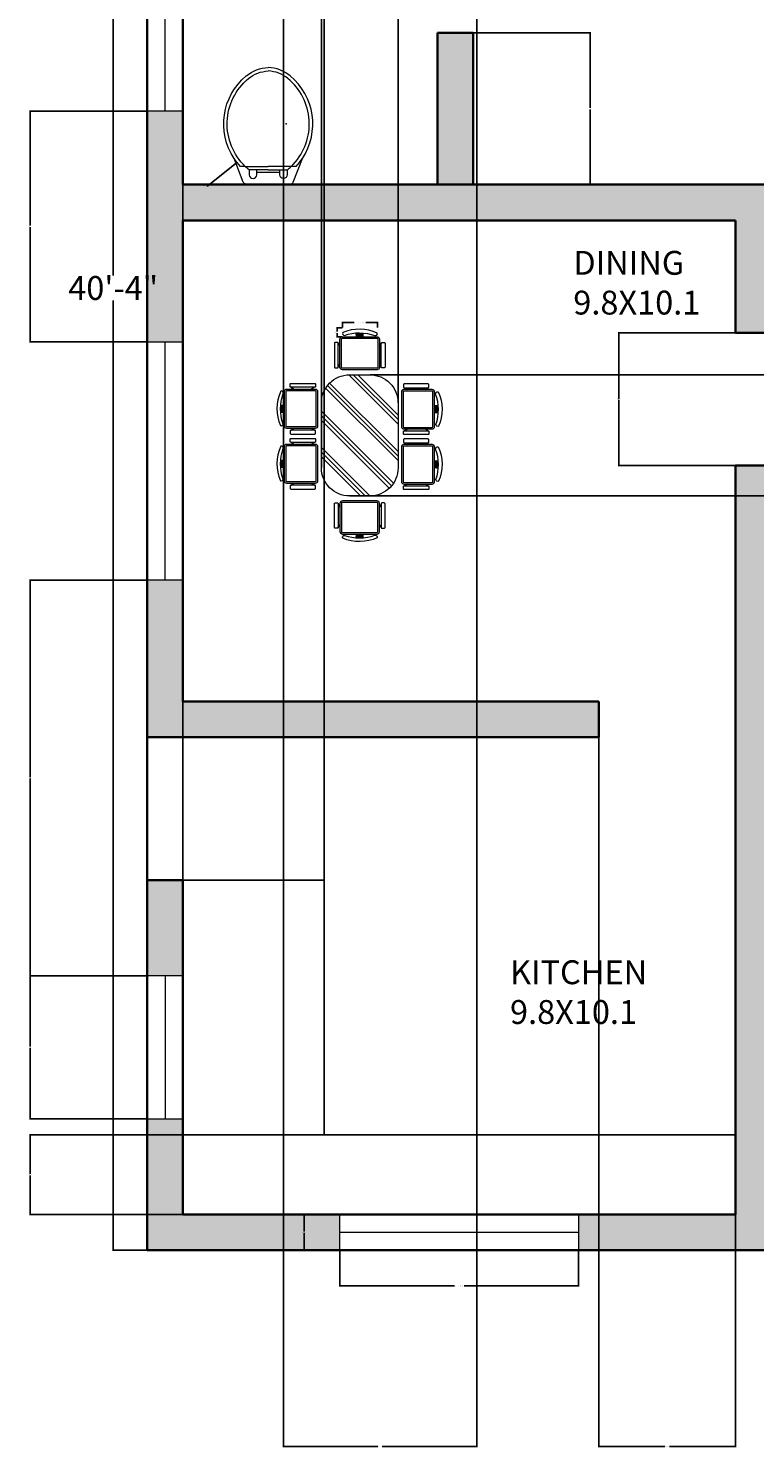
# Model space of a CAD drawing. Units: inches. Extents: x 0 to 423, y -517 to 94.
# Tile 1 of 8: x 0 to 182, y -517 to -160. Entities that reach past the tile are written whole.
import ezdxf

# ---------------------------------------------------------------- set-up
doc = ezdxf.new("R2010")
doc.units = ezdxf.units.IN
doc.header["$MEASUREMENT"] = 0
for name, color, linetype, lineweight in [('A-ANNO-DIMS', 2, 'Continuous', 18), ('A-AREA-IDEN', 7, 'Continuous', 18), ('A-FLOR-CASE', 8, 'Continuous', 25), ('A-FURN', 8, 'Continuous', 13), ('A-FURN-PATT', 8, 'Continuous', 13), ('A-GLAZ', 4, 'Continuous', 18), ('A-WALL', 7, 'Continuous', 35), ('WC-Detail_dwgmodels.com', 251, 'Continuous', 13), ('WC-Outline_dwgmodels.com', 250, 'Continuous', 18)]:
    doc.layers.add(name, color=color, linetype=linetype, lineweight=lineweight)
doc.layers.add('A-WALL-PATT', color=30, linetype='Continuous', lineweight=13, true_color=0xf26722)
doc.styles.get("Standard").update_dxf_attribs({"font": 'arial.ttf'})
doc.dimstyles.get("Standard").update_dxf_attribs({"dimtxt": 0.18, "dimasz": 0.18, "dimexe": 0.18, "dimexo": 0.0625, "dimgap": 0.09, "dimtad": 0, "dimtih": 1, "dimtoh": 1, "dimdec": 0, "dimzin": 0, "dimdsep": 46, "dimlunit": 3, "dimtxsty": 'Standard', "dimcen": 0.09, "dimadec": 0, "dimazin": 0, "dimtfac": 1, "dimtdec": 0, "dimtofl": 0, "dimtmove": 0, "dimatfit": 3, "dimfxl": 1, "dimtolj": 1, "dimtzin": 0, "dimarcsym": 0})

# ---------------------------------------------------------------- blocks, each defined once
blk = doc.blocks.new('*D2')
at = {"layer": 'A-ANNO-DIMS', "color": 0, "lineweight": -2, "transparency": 16777216}
for p, q in [((29.66, 16.23), (21, 16.23)), ((21.18, 16.05), (21.18, -222.61)), ((21.18, -467.59), (21.18, -228.92)), ((29.66, -467.77), (21, -467.77))]:
    blk.add_line(p, q, dxfattribs=at)
at = {"layer": 'A-ANNO-DIMS', "color": 0, "transparency": 16777216}
for points in [[(21.15, 16.05), (21.21, 16.05), (21.18, 16.23)], [(21.15, -467.59), (21.21, -467.59), (21.18, -467.77)]]:
    blk.add_solid(points, dxfattribs=at)
at = {"layer": 'Defpoints', "color": 0, "transparency": 16777216}
for p in [(29.72, 16.23), (21.18, -467.77), (29.72, -467.77)]:
    blk.add_point(p, dxfattribs=at)
at = {"layer": 'A-ANNO-DIMS', "color": 0, "transparency": 16777216, "insert": (21.18, -225.77), "char_height": 6, "attachment_point": 5}
blk.add_mtext('\\A1;40\'-4"', dxfattribs=at)
blk = doc.blocks.new('WIN-GLAZ-60IN')
for p, q in [((0, 60), (0, 0)), ((4.5, 60), (4.5, 0)), ((9, 0), (9, 60))]:
    blk.add_line(p, q)
blk = doc.blocks.new('WIN-GLAZ-24IN')
for p, q in [((0, 0), (0, 24)), ((4.5, 0), (4.5, 24)), ((9, 24), (9, 0))]:
    blk.add_line(p, q)
blk = doc.blocks.new('DINING-CHAIR-BACKREST')
for p, q in [((3.29, 0.7), (5.3, 0.7)), ((3.31, 0.47), (5.3, 0.47)), ((3.31, 0.2), (5.3, 0.2))]:
    blk.add_line(p, q)
blk.add_lwpolyline([(0.05, 1.03, 0.552014), (0.46, 0.34, -0.175809), (8.12, 0.28, 0.578392), (8.7, 0.92, 0.214524)], format="xyb", close=True)
blk.add_lwpolyline([(4.3, 0), (4.3, 0.93)])
blk = doc.blocks.new('*D12')
at = {"layer": 'A-ANNO-DIMS', "color": 0, "lineweight": -2, "transparency": 16777216}
for p, q in [((78.22, -467.83), (78.22, -476.95)), ((138.22, -467.83), (138.22, -476.95)), ((78.4, -476.77), (106.99, -476.77)), ((138.04, -476.77), (109.45, -476.77))]:
    blk.add_line(p, q, dxfattribs=at)
at = {"layer": 'A-ANNO-DIMS', "color": 0, "transparency": 16777216}
for points in [[(78.4, -476.74), (78.4, -476.8), (78.22, -476.77)], [(138.04, -476.74), (138.04, -476.8), (138.22, -476.77)]]:
    blk.add_solid(points, dxfattribs=at)
at = {"layer": 'Defpoints', "color": 0, "transparency": 16777216}
for p in [(78.22, -467.77), (138.22, -467.77), (78.22, -476.77)]:
    blk.add_point(p, dxfattribs=at)
at = {"layer": 'A-ANNO-DIMS', "color": 0, "transparency": 16777216, "insert": (108.22, -476.77), "char_height": 0.18, "attachment_point": 5}
blk.add_mtext('\\A1;WINDOW 5\'-0" TYP.', dxfattribs=at)
blk = doc.blocks.new('*D13')
at = {"layer": 'A-ANNO-DIMS', "color": 0, "lineweight": -2, "transparency": 16777216}
for p, q in [((78.16, -458.77), (69.04, -458.77)), ((69.22, -458.95), (69.22, -463.08)), ((69.22, -467.59), (69.22, -463.45)), ((78.16, -467.77), (69.04, -467.77))]:
    blk.add_line(p, q, dxfattribs=at)
at = {"layer": 'A-ANNO-DIMS', "color": 0, "transparency": 16777216}
for points in [[(69.19, -458.95), (69.25, -458.95), (69.22, -458.77)], [(69.19, -467.59), (69.25, -467.59), (69.22, -467.77)]]:
    blk.add_solid(points, dxfattribs=at)
at = {"layer": 'Defpoints', "color": 0, "transparency": 16777216}
for p in [(69.22, -458.77), (78.22, -458.77), (78.22, -467.77)]:
    blk.add_point(p, dxfattribs=at)
at = {"layer": 'A-ANNO-DIMS', "color": 0, "transparency": 16777216, "insert": (69.22, -463.27), "char_height": 0.18, "attachment_point": 5}
blk.add_mtext('\\A1;0\'-9" TYP.', dxfattribs=at)
blk = doc.blocks.new('*D16')
at = {"layer": 'A-ANNO-DIMS', "color": 0, "lineweight": -2, "transparency": 16777216}
for p, q in [((78.85, -235.73), (78.85, -234.3)), ((79.03, -234.48), (81.8, -234.48)), ((87.45, -234.48), (84.68, -234.48)), ((87.63, -235.73), (87.63, -234.3))]:
    blk.add_line(p, q, dxfattribs=at)
at = {"layer": 'A-ANNO-DIMS', "color": 0, "transparency": 16777216}
for points in [[(79.03, -234.45), (79.03, -234.51), (78.85, -234.48)], [(87.45, -234.45), (87.45, -234.51), (87.63, -234.48)]]:
    blk.add_solid(points, dxfattribs=at)
at = {"layer": 'Defpoints', "color": 0, "transparency": 16777216}
for p in [(87.63, -234.48), (78.85, -235.8), (87.63, -235.8)]:
    blk.add_point(p, dxfattribs=at)
at = {"layer": 'A-ANNO-DIMS', "color": 0, "transparency": 16777216, "insert": (83.24, -234.48), "char_height": 0.18, "attachment_point": 5}
blk.add_mtext('\\A1;CHAIR BACK 0\'-9" TYP.', dxfattribs=at)
blk = doc.blocks.new('*D17')
at = {"layer": 'A-ANNO-DIMS', "color": 0, "lineweight": -2, "transparency": 16777216}
for p, q in [((78.79, -235.8), (77.36, -235.8)), ((78.79, -238.03), (77.36, -238.03)), ((77.54, -235.98), (77.54, -236.73)), ((77.54, -237.85), (77.54, -237.09))]:
    blk.add_line(p, q, dxfattribs=at)
at = {"layer": 'A-ANNO-DIMS', "color": 0, "transparency": 16777216}
for points in [[(77.51, -235.98), (77.57, -235.98), (77.54, -235.8)], [(77.51, -237.85), (77.57, -237.85), (77.54, -238.03)]]:
    blk.add_solid(points, dxfattribs=at)
at = {"layer": 'Defpoints', "color": 0, "transparency": 16777216}
for p in [(77.54, -235.8), (78.85, -235.8), (78.85, -238.03)]:
    blk.add_point(p, dxfattribs=at)
at = {"layer": 'A-ANNO-DIMS', "color": 0, "transparency": 16777216, "insert": (77.54, -236.91), "char_height": 0.18, "attachment_point": 5}
blk.add_mtext('\\A1;0\'-2" TYP.', dxfattribs=at)
blk = doc.blocks.new('*D33')
at = {"layer": 'A-ANNO-DIMS', "color": 0, "lineweight": -2, "transparency": 16777216}
for p, q in [((38.72, -374.65), (38.72, 45.81)), ((38.9, 45.63), (55.89, 45.63)), ((74.1, 45.63), (57.11, 45.63)), ((74.28, -374.65), (74.28, 45.81))]:
    blk.add_line(p, q, dxfattribs=at)
at = {"layer": 'A-ANNO-DIMS', "color": 0, "transparency": 16777216}
for points in [[(38.9, 45.66), (38.9, 45.6), (38.72, 45.63)], [(74.1, 45.66), (74.1, 45.6), (74.28, 45.63)]]:
    blk.add_solid(points, dxfattribs=at)
at = {"layer": 'Defpoints', "color": 0, "transparency": 16777216}
for p in [(74.28, 45.63), (38.72, -374.71), (74.28, -374.71)]:
    blk.add_point(p, dxfattribs=at)
at = {"layer": 'A-ANNO-DIMS', "color": 0, "transparency": 16777216, "insert": (56.5, 45.63), "char_height": 0.18, "attachment_point": 5}
blk.add_mtext('\\A1;2\'-11 1/2"', dxfattribs=at)
blk = doc.blocks.new('*D34')
at = {"layer": 'A-ANNO-DIMS', "color": 0, "lineweight": -2, "transparency": 16777216}
for p, q in [((74.21, -438.77), (0.14, -438.77)), ((0.32, -438.95), (0.32, -448.59)), ((0.32, -458.59), (0.32, -448.95)), ((38.66, -458.77), (0.14, -458.77))]:
    blk.add_line(p, q, dxfattribs=at)
at = {"layer": 'A-ANNO-DIMS', "color": 0, "transparency": 16777216}
for points in [[(0.29, -438.95), (0.35, -438.95), (0.32, -438.77)], [(0.29, -458.59), (0.35, -458.59), (0.32, -458.77)]]:
    blk.add_solid(points, dxfattribs=at)
at = {"layer": 'Defpoints', "color": 0, "transparency": 16777216}
for p in [(0.32, -438.77), (74.28, -438.77), (38.72, -458.77)]:
    blk.add_point(p, dxfattribs=at)
at = {"layer": 'A-ANNO-DIMS', "color": 0, "transparency": 16777216, "insert": (0.32, -448.77), "char_height": 0.18, "attachment_point": 5}
blk.add_mtext('\\A1;1\'-8"', dxfattribs=at)
blk = doc.blocks.new('*D46')
at = {"layer": 'A-ANNO-DIMS', "color": 0, "lineweight": -2, "transparency": 16777216}
for p, q in [((29.66, -181.27), (0.14, -181.27)), ((0.32, -181.45), (0.32, -210.08)), ((0.32, -239.09), (0.32, -210.45)), ((29.66, -239.27), (0.14, -239.27))]:
    blk.add_line(p, q, dxfattribs=at)
at = {"layer": 'A-ANNO-DIMS', "color": 0, "transparency": 16777216}
for points in [[(0.29, -181.45), (0.35, -181.45), (0.32, -181.27)], [(0.29, -239.09), (0.35, -239.09), (0.32, -239.27)]]:
    blk.add_solid(points, dxfattribs=at)
at = {"layer": 'Defpoints', "color": 0, "transparency": 16777216}
for p in [(0.32, -181.27), (29.72, -181.27), (29.72, -239.27)]:
    blk.add_point(p, dxfattribs=at)
at = {"layer": 'A-ANNO-DIMS', "color": 0, "transparency": 16777216, "insert": (0.32, -210.27), "char_height": 0.18, "attachment_point": 5}
blk.add_mtext('\\A1;4\'-10"', dxfattribs=at)
blk = doc.blocks.new('*D47')
at = {"layer": 'A-ANNO-DIMS', "color": 0, "lineweight": -2, "transparency": 16777216}
for p, q in [((29.66, -299.27), (0.14, -299.27)), ((0.32, -299.45), (0.32, -348.82)), ((0.32, -398.56), (0.32, -349.18)), ((29.66, -398.74), (0.14, -398.74))]:
    blk.add_line(p, q, dxfattribs=at)
at = {"layer": 'A-ANNO-DIMS', "color": 0, "transparency": 16777216}
for points in [[(0.29, -299.45), (0.35, -299.45), (0.32, -299.27)], [(0.29, -398.56), (0.35, -398.56), (0.32, -398.74)]]:
    blk.add_solid(points, dxfattribs=at)
at = {"layer": 'Defpoints', "color": 0, "transparency": 16777216}
for p in [(0.32, -299.27), (29.72, -299.27), (29.72, -398.74)]:
    blk.add_point(p, dxfattribs=at)
at = {"layer": 'A-ANNO-DIMS', "color": 0, "transparency": 16777216, "insert": (0.32, -349), "char_height": 0.18, "attachment_point": 5}
blk.add_mtext('\\A1;8\'-3 1/2"', dxfattribs=at)
blk = doc.blocks.new('*D48')
at = {"layer": 'A-ANNO-DIMS', "color": 0, "lineweight": -2, "transparency": 16777216}
for p, q in [((29.66, -398.74), (0.14, -398.74)), ((0.32, -398.92), (0.32, -416.55)), ((0.32, -434.56), (0.32, -416.92)), ((29.66, -434.74), (0.14, -434.74))]:
    blk.add_line(p, q, dxfattribs=at)
at = {"layer": 'A-ANNO-DIMS', "color": 0, "transparency": 16777216}
for points in [[(0.29, -398.92), (0.35, -398.92), (0.32, -398.74)], [(0.29, -434.56), (0.35, -434.56), (0.32, -434.74)]]:
    blk.add_solid(points, dxfattribs=at)
at = {"layer": 'Defpoints', "color": 0, "transparency": 16777216}
for p in [(0.32, -398.74), (29.72, -398.74), (29.72, -434.74)]:
    blk.add_point(p, dxfattribs=at)
at = {"layer": 'A-ANNO-DIMS', "color": 0, "transparency": 16777216, "insert": (0.32, -416.74), "char_height": 0.18, "attachment_point": 5}
blk.add_mtext('\\A1;3\'-0"', dxfattribs=at)
blk = doc.blocks.new('*D49')
at = {"layer": 'A-ANNO-DIMS', "color": 0, "lineweight": -2, "transparency": 16777216}
for p, q in [((63.98, -61.2), (63.98, -517.35)), ((112.6, -61.2), (112.6, -517.35)), ((64.16, -517.17), (87.75, -517.17)), ((112.42, -517.17), (88.83, -517.17))]:
    blk.add_line(p, q, dxfattribs=at)
at = {"layer": 'A-ANNO-DIMS', "color": 0, "transparency": 16777216}
for points in [[(64.16, -517.14), (64.16, -517.2), (63.98, -517.17)], [(112.42, -517.14), (112.42, -517.2), (112.6, -517.17)]]:
    blk.add_solid(points, dxfattribs=at)
at = {"layer": 'Defpoints', "color": 0, "transparency": 16777216}
for p in [(63.98, -61.14), (112.6, -61.14), (112.6, -517.17)]:
    blk.add_point(p, dxfattribs=at)
at = {"layer": 'A-ANNO-DIMS', "color": 0, "transparency": 16777216, "insert": (88.29, -517.17), "char_height": 0.18, "attachment_point": 5}
blk.add_mtext('\\A1;4\'-0 1/2"', dxfattribs=at)
blk = doc.blocks.new('*D52')
at = {"layer": 'A-ANNO-DIMS', "color": 0, "lineweight": -2, "transparency": 16777216}
for p, q in [((73.55, -270.94), (73.55, 45.81)), ((73.73, 45.63), (82.66, 45.63)), ((92.66, 45.63), (83.72, 45.63)), ((92.84, -254.62), (92.84, 45.81))]:
    blk.add_line(p, q, dxfattribs=at)
at = {"layer": 'A-ANNO-DIMS', "color": 0, "transparency": 16777216}
for points in [[(73.73, 45.66), (73.73, 45.6), (73.55, 45.63)], [(92.66, 45.66), (92.66, 45.6), (92.84, 45.63)]]:
    blk.add_solid(points, dxfattribs=at)
at = {"layer": 'Defpoints', "color": 0, "transparency": 16777216}
for p in [(92.84, 45.63), (92.84, -254.68), (73.55, -271)]:
    blk.add_point(p, dxfattribs=at)
at = {"layer": 'A-ANNO-DIMS', "color": 0, "transparency": 16777216, "insert": (83.19, 45.63), "char_height": 0.18, "attachment_point": 5}
blk.add_mtext('\\A1;1\'-7 1/2"', dxfattribs=at)
blk = doc.blocks.new('*D53')
at = {"layer": 'A-ANNO-DIMS', "color": 0, "lineweight": -2, "transparency": 16777216}
for p, q in [((85.83, -247.61), (422.3, -247.61)), ((422.12, -247.79), (422.12, -262.66)), ((422.12, -277.89), (422.12, -263.02)), ((80.68, -278.07), (422.3, -278.07))]:
    blk.add_line(p, q, dxfattribs=at)
at = {"layer": 'A-ANNO-DIMS', "color": 0, "transparency": 16777216}
for points in [[(422.09, -247.79), (422.15, -247.79), (422.12, -247.61)], [(422.09, -277.89), (422.15, -277.89), (422.12, -278.07)]]:
    blk.add_solid(points, dxfattribs=at)
at = {"layer": 'Defpoints', "color": 0, "transparency": 16777216}
for p in [(85.77, -247.61), (80.61, -278.07), (422.12, -278.07)]:
    blk.add_point(p, dxfattribs=at)
at = {"layer": 'A-ANNO-DIMS', "color": 0, "transparency": 16777216, "insert": (422.12, -262.84), "char_height": 0.18, "attachment_point": 5}
blk.add_mtext('\\A1;2\'-6 1/2"', dxfattribs=at)
blk = doc.blocks.new('*D54')
at = {"layer": 'A-ANNO-DIMS', "color": 0, "lineweight": -2, "transparency": 16777216}
for p, q in [((177.72, -270.44), (177.72, -517.35)), ((143.29, -338.83), (143.29, -517.35)), ((143.47, -517.17), (159.9, -517.17)), ((177.54, -517.17), (161.12, -517.17))]:
    blk.add_line(p, q, dxfattribs=at)
at = {"layer": 'A-ANNO-DIMS', "color": 0, "transparency": 16777216}
for points in [[(143.47, -517.14), (143.47, -517.2), (143.29, -517.17)], [(177.54, -517.14), (177.54, -517.2), (177.72, -517.17)]]:
    blk.add_solid(points, dxfattribs=at)
at = {"layer": 'Defpoints', "color": 0, "transparency": 16777216}
for p in [(177.72, -270.38), (143.29, -338.77), (177.72, -517.17)]:
    blk.add_point(p, dxfattribs=at)
at = {"layer": 'A-ANNO-DIMS', "color": 0, "transparency": 16777216, "insert": (160.51, -517.17), "char_height": 0.18, "attachment_point": 5}
blk.add_mtext('\\A1;2\'-10 1/2"', dxfattribs=at)
blk = doc.blocks.new('*D56')
at = {"layer": 'A-ANNO-DIMS', "color": 0, "lineweight": -2, "transparency": 16777216}
for p, q in [((177.66, -237.07), (148.14, -237.07)), ((148.32, -237.25), (148.32, -253.54)), ((148.32, -270.2), (148.32, -253.91)), ((177.66, -270.38), (148.14, -270.38))]:
    blk.add_line(p, q, dxfattribs=at)
at = {"layer": 'A-ANNO-DIMS', "color": 0, "transparency": 16777216}
for points in [[(148.29, -237.25), (148.35, -237.25), (148.32, -237.07)], [(148.29, -270.2), (148.35, -270.2), (148.32, -270.38)]]:
    blk.add_solid(points, dxfattribs=at)
at = {"layer": 'Defpoints', "color": 0, "transparency": 16777216}
for p in [(148.32, -237.07), (177.72, -237.07), (177.72, -270.38)]:
    blk.add_point(p, dxfattribs=at)
at = {"layer": 'A-ANNO-DIMS', "color": 0, "transparency": 16777216, "insert": (148.32, -253.72), "char_height": 0.18, "attachment_point": 5}
blk.add_mtext('\\A1;2\'-9 1/2"', dxfattribs=at)
blk = doc.blocks.new('*D57')
at = {"layer": 'A-ANNO-DIMS', "color": 0, "lineweight": -2, "transparency": 16777216}
for p, q in [((111.79, -161.55), (141.3, -161.55)), ((141.12, -161.73), (141.12, -180.47)), ((141.12, -199.59), (141.12, -180.84)), ((111.79, -199.77), (141.3, -199.77))]:
    blk.add_line(p, q, dxfattribs=at)
at = {"layer": 'A-ANNO-DIMS', "color": 0, "transparency": 16777216}
for points in [[(141.09, -161.73), (141.15, -161.73), (141.12, -161.55)], [(141.09, -199.59), (141.15, -199.59), (141.12, -199.77)]]:
    blk.add_solid(points, dxfattribs=at)
at = {"layer": 'Defpoints', "color": 0, "transparency": 16777216}
for p in [(111.72, -161.55), (111.72, -199.77), (141.12, -199.77)]:
    blk.add_point(p, dxfattribs=at)
at = {"layer": 'A-ANNO-DIMS', "color": 0, "transparency": 16777216, "insert": (141.12, -180.66), "char_height": 0.18, "attachment_point": 5}
blk.add_mtext('\\A1;3\'-2"', dxfattribs=at)
blk = doc.blocks.new('*D67')
at = {"layer": 'A-ANNO-DIMS', "color": 0, "lineweight": -2, "transparency": 16777216}
for p, q in [((64.56, -184.51), (64.74, -184.51)), ((64.65, -184.6), (64.65, -184.42)), ((44.95, -200.04), (52.2, -194.33)), ((44.77, -200.04), (44.95, -200.04))]:
    blk.add_line(p, q, dxfattribs=at)
at = {"layer": 'A-ANNO-DIMS', "color": 0, "transparency": 16777216}
blk.add_solid([(52.18, -194.31), (52.22, -194.35), (52.34, -194.22)], dxfattribs=at)
at = {"layer": 'Defpoints', "color": 0, "transparency": 16777216}
for p in [(64.65, -184.51), (52.34, -194.22)]:
    blk.add_point(p, dxfattribs=at)
at = {"layer": 'A-ANNO-DIMS', "color": 0, "transparency": 16777216, "insert": (44.15, -200.04), "char_height": 0.18, "attachment_point": 5}
blk.add_mtext('\\A1;R1\'-3 1/2"', dxfattribs=at)

msp = doc.modelspace()

# ---------------------------------------------------------------- hatches: boundary and pattern name
at = {"layer": 'A-FURN-PATT'}
h = msp.add_hatch(dxfattribs=at)
h.set_pattern_fill('PLAST', color=256, scale=25.912, angle=135, style=0)
h.paths.add_polyline_path([(85.77, -278.07), (80.61, -278.07), (80.25, -278.06), (79.89, -278.03), (79.54, -277.98), (79.19, -277.92), (78.85, -277.84), (78.51, -277.75), (78.18, -277.64), (77.86, -277.51), (77.55, -277.37), (77.25, -277.21), (76.95, -277.04), (76.66, -276.86), (76.39, -276.66), (76.12, -276.45), (75.86, -276.23), (75.62, -276), (75.38, -275.75), (75.16, -275.49), (74.95, -275.23), (74.75, -274.95), (74.57, -274.66), (74.4, -274.37), (74.24, -274.06), (74.1, -273.75), (73.98, -273.43), (73.87, -273.1), (73.77, -272.77), (73.69, -272.42), (73.63, -272.08), (73.58, -271.72), (73.56, -271.36), (73.55, -271), (73.55, -254.68), (73.56, -254.32), (73.58, -253.96), (73.63, -253.6), (73.69, -253.25), (73.77, -252.91), (73.87, -252.58), (73.98, -252.25), (74.1, -251.93), (74.24, -251.61), (74.4, -251.31), (74.57, -251.01), (74.75, -250.73), (74.95, -250.45), (75.16, -250.18), (75.38, -249.93), (75.62, -249.68), (75.86, -249.45), (76.12, -249.23), (76.39, -249.02), (76.66, -248.82), (76.95, -248.63), (77.25, -248.46), (77.55, -248.31), (77.86, -248.17), (78.18, -248.04), (78.51, -247.93), (78.85, -247.83), (79.19, -247.76), (79.54, -247.69), (79.89, -247.65), (80.25, -247.62), (80.61, -247.61), (85.77, -247.61), (86.13, -247.62), (86.49, -247.65), (86.85, -247.69), (87.2, -247.76), (87.54, -247.83), (87.87, -247.93), (88.2, -248.04), (88.52, -248.17), (88.83, -248.31), (89.14, -248.46), (89.44, -248.63), (89.72, -248.82), (90, -249.02), (90.27, -249.23), (90.52, -249.45), (90.77, -249.68), (91, -249.93), (91.22, -250.18), (91.43, -250.45), (91.63, -250.73), (91.81, -251.01), (91.99, -251.31), (92.14, -251.61), (92.28, -251.93), (92.41, -252.25), (92.52, -252.58), (92.62, -252.91), (92.69, -253.25), (92.76, -253.6), (92.8, -253.96), (92.83, -254.32), (92.84, -254.68), (92.84, -271), (92.83, -271.35), (92.8, -271.7), (92.76, -272.04), (92.7, -272.38), (92.62, -272.72), (92.53, -273.05), (92.42, -273.38), (92.3, -273.7), (92.16, -274.02), (92.01, -274.33), (91.84, -274.63), (91.65, -274.92), (91.45, -275.2), (91.24, -275.48), (91.01, -275.74), (90.77, -276), (90.51, -276.24), (90.25, -276.47), (89.98, -276.68), (89.69, -276.88), (89.4, -277.06), (89.1, -277.23), (88.79, -277.39), (88.48, -277.53), (88.15, -277.65), (87.83, -277.76), (87.49, -277.85), (87.16, -277.93), (86.81, -277.99), (86.47, -278.03), (86.12, -278.06)])
at = {"layer": 'A-WALL-PATT'}
h = msp.add_hatch(color=256, dxfattribs=at)
h.dxf.hatch_style = 1
h.paths.add_polyline_path([(201.52, 16.23), (138.22, 16.23), (138.22, 7.23), (177.72, 7.23), (177.72, -138.77), (186.72, -138.77), (186.72, -92.77), (251.72, -92.77), (251.72, -22.53), (242.72, -22.53), (242.72, -83.77), (186.72, -83.77), (186.72, 7.23), (201.52, 7.23)])
h.paths.add_polyline_path([(78.22, 16.23), (29.72, 16.23), (29.72, -31.27), (38.72, -31.27), (38.72, 7.23), (78.22, 7.23)])
h.paths.add_polyline_path([(275.31, 16.23), (225.52, 16.23), (225.52, 7.23), (275.31, 7.23)])
h.paths.add_polyline_path([(392.72, 16.23), (335.31, 16.23), (335.31, 7.23), (383.72, 7.23), (383.72, -31.27), (392.72, -31.27)])
h.paths.add_polyline_path([(143.33, -129.77), (38.72, -129.77), (38.72, -91.27), (29.72, -91.27), (29.72, -157.27), (38.72, -157.27), (38.72, -138.77), (143.33, -138.77)])
h.paths.add_polyline_path([(186.72, -199.77), (38.72, -199.77), (38.72, -181.27), (29.72, -181.27), (29.72, -239.27), (38.72, -239.27), (38.72, -208.77), (177.72, -208.77), (177.72, -237.07), (186.72, -237.07)])
h.paths.add_polyline_path([(111.72, -161.55), (102.72, -161.55), (102.72, -199.77), (111.72, -199.77)])
h.paths.add_polyline_path([(392.72, -91.27), (383.72, -91.27), (383.72, -129.77), (242.72, -129.77), (242.72, -138.77), (383.72, -138.77), (383.72, -169.77), (392.72, -169.77)])
h.paths.add_polyline_path([(392.72, -229.77), (383.72, -229.77), (383.72, -262.77), (251.72, -262.77), (251.72, -177.14), (242.72, -177.14), (242.72, -271.77), (383.72, -271.77), (383.72, -300.77), (392.72, -300.77)])
h.paths.add_polyline_path([(392.72, -360.77), (383.72, -360.77), (383.72, -389.77), (378.42, -389.77), (378.42, -398.77), (383.72, -398.77), (383.72, -458.77), (382.72, -458.77), (382.72, -467.77), (392.72, -467.77)])
h.paths.add_polyline_path([(364.92, -389.77), (348.72, -389.77), (348.72, -467.77), (358.72, -467.77), (358.72, -458.77), (357.72, -458.77), (357.72, -398.77), (364.92, -398.77)])
h.paths.add_polyline_path([(320.72, -389.77), (283.72, -389.77), (283.72, -398.77), (320.72, -398.77)])
h.paths.add_polyline_path([(223.72, -389.77), (186.72, -389.77), (186.72, -270.38), (177.72, -270.38), (177.72, -458.77), (138.22, -458.77), (138.22, -467.77), (186.72, -467.77), (186.72, -398.77), (223.72, -398.77)])
h.paths.add_polyline_path([(143.29, -329.77), (38.72, -329.77), (38.72, -299.27), (29.72, -299.27), (29.72, -338.77), (143.29, -338.77)])
h.paths.add_polyline_path([(38.72, -374.71), (29.72, -374.71), (29.72, -398.74), (38.72, -398.74)])
h.paths.add_polyline_path([(78.22, -458.77), (38.72, -458.77), (38.72, -434.74), (29.72, -434.74), (29.72, -467.77), (78.22, -467.77)])
h.paths.add_polyline_path([(279.99, -158.17), (326.6, -158.17), (326.6, -135.78), (279.99, -135.78)], flags=25)
h.paths.add_polyline_path([(355.56, -439.13), (387, -439.13), (387, -416.66), (355.56, -416.66)], flags=9)

# ---------------------------------------------------------------- linework, layer by layer
at = {"layer": 'A-FLOR-CASE'}
for p, q in [((38.72, -374.71), (74.28, -374.71)), ((74.28, -374.71), (74.28, -438.77)), ((74.28, -438.77), (177.72, -438.77))]:
    msp.add_line(p, q, dxfattribs=at)
at = {"layer": 'A-FURN'}
for p, q in [((77.79, -239.74), (78.21, -240.26)), ((88.57, -239.74), (88.14, -240.26)), ((77.79, -245.58), (78.21, -244.88)), ((88.57, -245.58), (88.14, -244.88)), ((65.96, -250.74), (66.48, -251.17)), ((71.8, -250.74), (71.1, -251.17)), ((94.45, -250.88), (95.15, -251.31)), ((100.29, -250.88), (99.76, -251.31)), ((65.96, -261.53), (66.48, -261.1)), ((71.8, -261.53), (71.1, -261.1)), ((94.45, -261.66), (95.15, -261.24)), ((100.29, -261.66), (99.76, -261.24)), ((65.96, -264.58), (66.48, -265.01)), ((71.8, -264.58), (71.1, -265.01)), ((94.45, -264.72), (95.15, -265.15)), ((100.29, -264.72), (99.76, -265.15)), ((65.96, -275.37), (66.48, -274.94)), ((71.8, -275.37), (71.1, -274.94)), ((94.45, -275.5), (95.15, -275.08)), ((100.29, -275.5), (99.76, -275.08)), ((77.79, -280.1), (78.21, -280.8)), ((88.57, -280.1), (88.14, -280.8)), ((77.79, -285.94), (78.21, -285.42)), ((88.57, -285.94), (88.14, -285.42))]:
    msp.add_line(p, q, dxfattribs=at)
for points in [[(88.13, -238.62), (88.13, -245.76, -0.414214), (87.54, -246.35), (78.82, -246.35, -0.414214), (78.22, -245.76), (78.22, -238.62, -0.414214), (78.82, -238.03)], [(78.82, -238.03), (87.54, -238.03, -0.414214), (88.13, -238.62)], [(89.35, -239.49, -0.414214), (89.55, -239.69), (89.55, -245.64, -0.414214), (89.35, -245.83), (88.76, -245.83, -0.414214), (88.56, -245.64), (88.56, -239.69, -0.414214)], [(88.56, -239.69, -0.414214), (88.76, -239.49), (89.35, -239.49, -0.414214)], [(65.71, -249.96, -0.414214), (65.91, -249.76), (71.86, -249.76, -0.414214), (72.06, -249.96), (72.06, -250.55, -0.414214), (71.86, -250.75), (65.91, -250.75, -0.414214)], [(64.84, -251.18), (71.98, -251.18, -0.414214), (72.58, -251.77), (72.58, -260.5, -0.414214), (71.98, -261.09), (64.84, -261.09, -0.414214), (64.25, -260.5)], [(64.25, -260.5), (64.25, -251.77, -0.414214), (64.84, -251.18)], [(65.91, -250.75, -0.414214), (65.71, -250.55), (65.71, -249.96, -0.414214)], [(102, -251.91, 0.414214), (101.4, -251.32), (94.27, -251.32, 0.414214), (93.67, -251.91), (93.67, -260.63, 0.414214), (94.27, -261.23), (101.4, -261.23, 0.414214), (102, -260.63)], [(100.54, -250.1, 0.414214), (100.34, -249.9), (94.39, -249.9, 0.414214), (94.19, -250.1), (94.19, -250.69, 0.414214), (94.39, -250.89), (100.34, -250.89, 0.414214)], [(100.34, -250.89, 0.414214), (100.54, -250.69), (100.54, -250.1, 0.414214)], [(102, -260.63), (102, -251.91, 0.414214)], [(65.71, -263.8, -0.414214), (65.91, -263.6), (71.86, -263.6, -0.414214), (72.06, -263.8), (72.06, -264.39, -0.414214), (71.86, -264.59), (65.91, -264.59, -0.414214)], [(65.91, -264.59, -0.414214), (65.71, -264.39), (65.71, -263.8, -0.414214)], [(100.54, -263.94, 0.414214), (100.34, -263.74), (94.39, -263.74, 0.414214), (94.19, -263.94), (94.19, -264.53, 0.414214), (94.39, -264.73), (100.34, -264.73, 0.414214)], [(100.34, -264.73, 0.414214), (100.54, -264.53), (100.54, -263.94, 0.414214)], [(64.84, -265.02), (71.98, -265.02, -0.414214), (72.58, -265.61), (72.58, -274.34, -0.414214), (71.98, -274.93), (64.84, -274.93, -0.414214), (64.25, -274.34)], [(64.25, -274.34), (64.25, -265.61, -0.414214), (64.84, -265.02)], [(102, -265.75, 0.414214), (101.4, -265.16), (94.27, -265.16, 0.414214), (93.67, -265.75), (93.67, -274.47, 0.414214), (94.27, -275.07), (101.4, -275.07, 0.414214), (102, -274.47)], [(102, -274.47), (102, -265.75, 0.414214)], [(87.54, -287.65, 0.414214), (88.13, -287.06), (88.13, -279.92, 0.414214), (87.54, -279.32), (78.82, -279.32, 0.414214), (78.22, -279.92), (78.22, -287.06, 0.414214), (78.82, -287.65)], [(89.35, -286.19, 0.414214), (89.55, -285.99), (89.55, -280.04, 0.414214), (89.35, -279.84), (88.76, -279.84, 0.414214), (88.56, -280.04), (88.56, -285.99, 0.414214)], [(78.82, -287.65), (87.54, -287.65, 0.414214)], [(88.56, -285.99, 0.414214), (88.76, -286.19), (89.35, -286.19, 0.414214)]]:
    msp.add_lwpolyline(points, format="xyb", dxfattribs=at)
for points in [[(78.82, -238.42), (87.54, -238.42, -0.414214), (87.74, -238.62), (87.74, -245.76, -0.414214), (87.54, -245.96), (78.82, -245.96, -0.414214), (78.62, -245.76), (78.62, -238.62, -0.414214)], [(77.6, -239.49), (77, -239.49, 0.414214), (76.8, -239.69), (76.8, -245.64, 0.414214), (77, -245.83), (77.6, -245.83, 0.414214), (77.79, -245.64), (77.79, -239.69, 0.414214)], [(85.77, -278.07), (80.61, -278.07, -0.414214), (73.55, -271), (73.55, -254.68, -0.414214), (80.61, -247.61), (85.77, -247.61, -0.414214), (92.84, -254.68), (92.84, -271, -0.414214)], [(64.65, -260.5), (64.65, -251.77, -0.414214), (64.84, -251.58), (71.98, -251.58, -0.414214), (72.18, -251.77), (72.18, -260.5, -0.414214), (71.98, -260.7), (64.84, -260.7, -0.414214)], [(101.6, -260.63), (101.6, -251.91, 0.414214), (101.4, -251.71), (94.27, -251.71, 0.414214), (94.07, -251.91), (94.07, -260.63, 0.414214), (94.27, -260.83), (101.4, -260.83, 0.414214)], [(65.71, -261.72), (65.71, -262.31, 0.414214), (65.91, -262.51), (71.86, -262.51, 0.414214), (72.06, -262.31), (72.06, -261.72, 0.414214), (71.86, -261.52), (65.91, -261.52, 0.414214)], [(100.54, -261.85), (100.54, -262.45, -0.414214), (100.34, -262.65), (94.39, -262.65, -0.414214), (94.19, -262.45), (94.19, -261.85, -0.414214), (94.39, -261.66), (100.34, -261.66, -0.414214)], [(64.65, -274.34), (64.65, -265.61, -0.414214), (64.84, -265.42), (71.98, -265.42, -0.414214), (72.18, -265.61), (72.18, -274.34, -0.414214), (71.98, -274.53), (64.84, -274.53, -0.414214)], [(101.6, -274.47), (101.6, -265.75, 0.414214), (101.4, -265.55), (94.27, -265.55, 0.414214), (94.07, -265.75), (94.07, -274.47, 0.414214), (94.27, -274.67), (101.4, -274.67, 0.414214)], [(65.71, -275.56), (65.71, -276.15, 0.414214), (65.91, -276.35), (71.86, -276.35, 0.414214), (72.06, -276.15), (72.06, -275.56, 0.414214), (71.86, -275.36), (65.91, -275.36, 0.414214)], [(100.54, -275.69), (100.54, -276.29, -0.414214), (100.34, -276.49), (94.39, -276.49, -0.414214), (94.19, -276.29), (94.19, -275.69, -0.414214), (94.39, -275.5), (100.34, -275.5, -0.414214)], [(77.6, -286.19), (77, -286.19, -0.414214), (76.8, -285.99), (76.8, -280.04, -0.414214), (77, -279.84), (77.6, -279.84, -0.414214), (77.79, -280.04), (77.79, -285.99, -0.414214)], [(78.82, -287.25), (87.54, -287.25, 0.414214), (87.74, -287.06), (87.74, -279.92, 0.414214), (87.54, -279.72), (78.82, -279.72, 0.414214), (78.62, -279.92), (78.62, -287.06, 0.414214)]]:
    msp.add_lwpolyline(points, format="xyb", close=True, dxfattribs=at)
for points in [[(77.59, -239.49), (78.22, -240.27)], [(88.13, -240.27), (88.56, -239.75)], [(78.22, -244.86), (77.79, -245.56)], [(88.56, -245.56), (88.13, -244.86)], [(66.5, -251.18), (65.97, -250.75)], [(71.78, -250.75), (71.08, -251.18)], [(94.46, -250.89), (95.17, -251.32)], [(99.75, -251.32), (100.28, -250.89)], [(65.71, -261.73), (66.5, -261.09)], [(71.08, -261.09), (71.78, -261.52)], [(95.17, -261.23), (94.46, -261.66)], [(100.54, -261.86), (99.75, -261.23)], [(66.5, -265.02), (65.97, -264.59)], [(71.78, -264.59), (71.08, -265.02)], [(94.46, -264.73), (95.17, -265.16)], [(99.75, -265.16), (100.28, -264.73)], [(65.71, -275.57), (66.5, -274.93)], [(71.08, -274.93), (71.78, -275.36)], [(95.17, -275.07), (94.46, -275.5)], [(100.54, -275.7), (99.75, -275.07)], [(78.22, -280.82), (77.79, -280.12)], [(88.56, -280.12), (88.13, -280.82)], [(77.59, -286.19), (78.22, -285.4)], [(88.13, -285.4), (88.56, -285.93)]]:
    msp.add_lwpolyline(points, dxfattribs=at)
at = {"layer": 'A-GLAZ'}
for p, q in [((38.72, -181.27), (29.72, -181.27)), ((29.72, -239.27), (38.72, -239.27)), ((38.72, -299.27), (29.72, -299.27)), ((29.72, -398.74), (29.72, -434.74)), ((38.72, -398.74), (29.72, -398.74)), ((34.22, -398.74), (34.22, -434.74)), ((38.72, -434.74), (38.72, -398.74)), ((29.72, -434.74), (38.72, -434.74)), ((78.22, -467.77), (78.22, -458.77)), ((138.22, -458.77), (138.22, -467.77))]:
    msp.add_line(p, q, dxfattribs=at)
at = {"layer": 'A-WALL'}
for p, q in [((29.72, 16.23), (29.72, -467.77)), ((38.72, -138.77), (38.72, -199.77)), ((102.72, -161.55), (102.72, -199.77)), ((102.72, -161.55), (111.72, -161.55)), ((111.72, -161.55), (111.72, -199.77)), ((38.72, -199.77), (186.72, -199.77)), ((38.72, -208.77), (177.72, -208.77)), ((38.72, -208.77), (38.72, -329.77)), ((177.72, -208.77), (177.72, -237.07)), ((177.72, -237.07), (186.72, -237.07)), ((186.72, -270.38), (177.72, -270.38)), ((177.72, -270.38), (177.72, -458.77)), ((38.72, -329.77), (143.29, -329.77)), ((143.29, -329.77), (143.29, -338.77)), ((29.72, -338.77), (143.29, -338.77)), ((38.72, -374.71), (29.72, -374.71)), ((38.72, -374.71), (38.72, -458.77)), ((38.72, -458.77), (177.72, -458.77)), ((29.72, -467.77), (392.72, -467.77))]:
    msp.add_line(p, q, dxfattribs=at)
at = {"layer": 'WC-Detail_dwgmodels.com'}
for p, q in [((54.4, -195.19), (53.17, -195.19)), ((67.17, -195.19), (65.94, -195.19))]:
    msp.add_line(p, q, dxfattribs=at)
for points in [[(53.17, -195.19, -0.040937), (51.59, -193.18, -0.163732)], [(55.41, -196.08, -0.022712), (54.4, -195.19, -0.162618)], [(60.17, -196.08), (55.41, -196.08, -0.476108)], [(55.41, -196.08), (55.41, -197.31, 1), (57.28, -197.31), (57.28, -196.67)], [(60.17, -196.08), (64.93, -196.08, 0.022712)], [(64.93, -196.08), (64.93, -197.31, -1), (63.06, -197.31), (63.06, -196.67)], [(64.93, -196.08, 0.022712), (65.94, -195.19, 0.162618)], [(67.17, -195.19, 0.040937), (68.76, -193.18, 0.163732)]]:
    msp.add_lwpolyline(points, format="xyb", dxfattribs=at)
for points in [[(57.28, -196.67), (57.28, -196.08)], [(63.06, -196.67), (63.06, -196.08)], [(57.28, -196.67), (63.06, -196.67)]]:
    msp.add_lwpolyline(points, dxfattribs=at)
at = {"layer": 'WC-Outline_dwgmodels.com'}
for p in [(54.4, -195.19), (65.94, -195.19)]:
    msp.add_line(p, (60.17, -195.19), dxfattribs=at)
for points in [[(51.59, -193.18, -0.383919), (54.66, -172.42, -0.163732), (60.17, -170.31, -0.359733)], [(54.4, -195.19, -0.448546), (55.22, -173.1, -0.162618), (60.17, -171.19, -0.470877)], [(68.76, -193.18, 0.383919), (65.68, -172.42, 0.163732), (60.17, -170.31, 0.359733)], [(66.53, -194.59, 0.431639), (65.12, -173.1, 0.162618), (60.17, -171.19, 0.470877)], [(60.17, -199.63), (54.57, -199.63, -0.31031), (53.89, -199.16), (51.59, -193.18, -0.209071)], [(60.17, -199.63), (65.77, -199.63, 0.31031), (66.46, -199.16), (68.76, -193.18, 0.209071)], [(65.94, -195.19, 0.014165), (66.53, -194.59, 0.162618)]]:
    msp.add_lwpolyline(points, format="xyb", dxfattribs=at)

# ---------------------------------------------------------------- block references
at = {"layer": 'A-FURN'}
msp.add_blockref('DINING-CHAIR-BACKREST', (78.87, -238.03), dxfattribs=at)
at = {"layer": 'A-FURN', "rotation": 90}
for p in [(64.25, -260.44), (64.25, -274.28)]:
    msp.add_blockref('DINING-CHAIR-BACKREST', p, dxfattribs=at)
at = {"layer": 'A-FURN', "extrusion": (0, 0, -1), "zscale": -1}
for p, rotation in [((-102, -260.58), 90), ((-102, -274.42), 90), ((-78.87, -287.65), 180)]:
    msp.add_blockref('DINING-CHAIR-BACKREST', p, dxfattribs=dict(at, rotation=rotation))
at = {"layer": 'A-GLAZ'}
msp.add_blockref('WIN-GLAZ-24IN', (29.72, -181.26), dxfattribs=at)
for p, rotation in [((38.72, -239.27), 180), ((138.22, -467.76), 90)]:
    msp.add_blockref('WIN-GLAZ-60IN', p, dxfattribs=dict(at, rotation=rotation))

# ---------------------------------------------------------------- texts
at = {"layer": 'A-AREA-IDEN', "char_height": 6, "attachment_point": 1}
for s, insert in [('DINING\\P9.8X10.1', (136.89, -216.44)), ('KITCHEN\\P9.8X10.1', (120.97, -394.87))]:
    msp.add_mtext(s, dxfattribs=dict(at, insert=insert))

# ---------------------------------------------------------------- dimensions: what is measured, and where the dimension line sits
at = {"layer": 'A-ANNO-DIMS'}
for base, p1, p2, picture, middle in [((74.28, 45.63), (38.72, -374.71), (74.28, -374.71), '*D33', (56.5, 45.63)), ((92.84, 45.63), (73.55, -271), (92.84, -254.68), '*D52', (83.19, 45.63)), ((112.6, -517.17), (63.98, -61.14), (112.6, -61.14), '*D49', (88.29, -517.17)), ((177.72, -517.17), (143.29, -338.77), (177.72, -270.38), '*D54', (160.51, -517.17))]:
    dim = msp.add_linear_dim(base=base, p1=p1, p2=p2, dimstyle='Standard', override={"dimdec": 1, "dimlfac": 1, "dimrnd": 0, "dimzin": 1, "dimdsep": 46, "dimlunit": 4, "dimfrac": 2}, dxfattribs=at)
    dim.commit()
    dim.dimension.update_dxf_attribs({"geometry": picture, "text_midpoint": middle})
for base, p1, p2, angle, override, picture, middle in [((21.18, -467.77), (29.72, 16.23), (29.72, -467.77), 90, {"dimtxt": 6, "dimclrd": 0, "dimclre": 0, "dimclrt": 0}, '*D2', (21.18, -225.77)), ((141.12, -199.77), (111.72, -161.55), (111.72, -199.77), 270, {"dimdec": 1, "dimlfac": 1, "dimrnd": 0, "dimzin": 1, "dimdsep": 46, "dimlunit": 4, "dimfrac": 2}, '*D57', (141.12, -180.66)), ((0.32, -181.27), (29.72, -239.27), (29.72, -181.27), 90, {"dimdec": 1, "dimlfac": 1, "dimrnd": 0, "dimzin": 1, "dimdsep": 46, "dimlunit": 4, "dimfrac": 2}, '*D46', (0.32, -210.27)), ((148.32, -237.07), (177.72, -270.38), (177.72, -237.07), 90, {"dimdec": 1, "dimlfac": 1, "dimrnd": 0, "dimzin": 1, "dimdsep": 46, "dimlunit": 4, "dimfrac": 2}, '*D56', (148.32, -253.72)), ((422.12, -278.07), (85.77, -247.61), (80.61, -278.07), 90, {"dimdec": 1, "dimlfac": 1, "dimrnd": 0, "dimzin": 1, "dimdsep": 46, "dimlunit": 4, "dimfrac": 2}, '*D53', (422.12, -262.84)), ((0.32, -299.27), (29.72, -398.74), (29.72, -299.27), 90, {"dimdec": 1, "dimlfac": 1, "dimrnd": 0, "dimzin": 1, "dimdsep": 46, "dimlunit": 4, "dimfrac": 2}, '*D47', (0.32, -349)), ((0.32, -398.74), (29.72, -434.74), (29.72, -398.74), 90, {"dimdec": 1, "dimlfac": 1, "dimrnd": 0, "dimzin": 1, "dimdsep": 46, "dimlunit": 4, "dimfrac": 2}, '*D48', (0.32, -416.74)), ((0.32, -438.77), (38.72, -458.77), (74.28, -438.77), 90, {"dimdec": 1, "dimlfac": 1, "dimrnd": 0, "dimzin": 1, "dimdsep": 46, "dimlunit": 4, "dimfrac": 2}, '*D34', (0.32, -448.77))]:
    dim = msp.add_linear_dim(base=base, p1=p1, p2=p2, angle=angle, dimstyle='Standard', override=override, dxfattribs=at)
    dim.commit()
    dim.dimension.update_dxf_attribs({"geometry": picture, "text_midpoint": middle})
dim = msp.add_radius_dim(center=(64.65, -184.51), mpoint=(52.34, -194.22), dimstyle='Standard', override={"dimdec": 1, "dimlfac": 1, "dimrnd": 0, "dimzin": 1, "dimdsep": 46, "dimlunit": 4, "dimfrac": 2}, dxfattribs=at)
dim.commit()
dim.dimension.update_dxf_attribs({"geometry": '*D67', "text_midpoint": (44.15, -200.04), "dimtype": 164})
dim = msp.add_linear_dim(base=(87.63, -234.48), p1=(78.85, -235.8), p2=(87.63, -235.8), text='CHAIR BACK <> TYP.', dimstyle='Standard', override={"dimdec": 1, "dimlfac": 1, "dimrnd": 0, "dimzin": 1, "dimdsep": 46, "dimlunit": 4, "dimfrac": 2}, dxfattribs=at)
dim.commit()
dim.dimension.update_dxf_attribs({"geometry": '*D16', "text_midpoint": (83.24, -234.48)})
for base, p1, p2, angle, text, picture, middle in [((77.54, -235.8), (78.85, -238.03), (78.85, -235.8), 90, '<> TYP.', '*D17', (77.54, -236.91)), ((69.22, -458.77), (78.22, -467.77), (78.22, -458.77), 90, '<> TYP.', '*D13', (69.22, -463.27)), ((78.22, -476.77), (138.22, -467.77), (78.22, -467.77), 180, 'WINDOW <> TYP.', '*D12', (108.22, -476.77))]:
    dim = msp.add_linear_dim(base=base, p1=p1, p2=p2, angle=angle, text=text, dimstyle='Standard', override={"dimdec": 1, "dimlfac": 1, "dimrnd": 0, "dimzin": 1, "dimdsep": 46, "dimlunit": 4, "dimfrac": 2}, dxfattribs=at)
    dim.commit()
    dim.dimension.update_dxf_attribs({"geometry": picture, "text_midpoint": middle})

doc.saveas('drawing.dxf')
